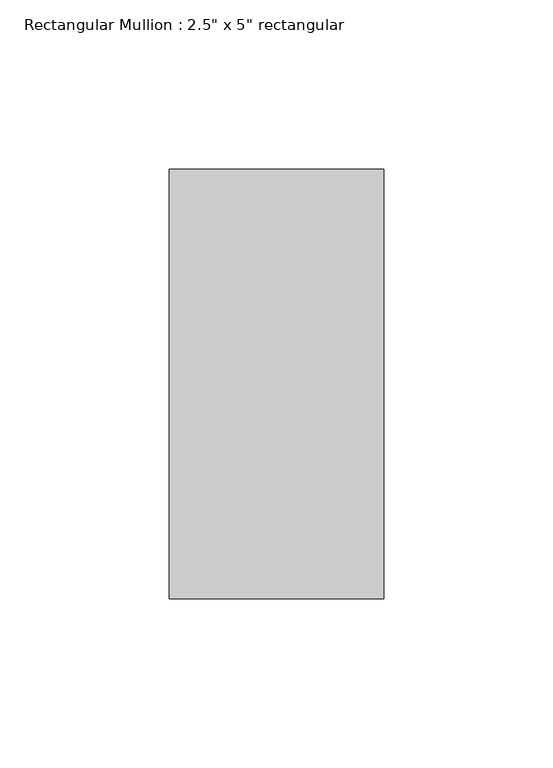
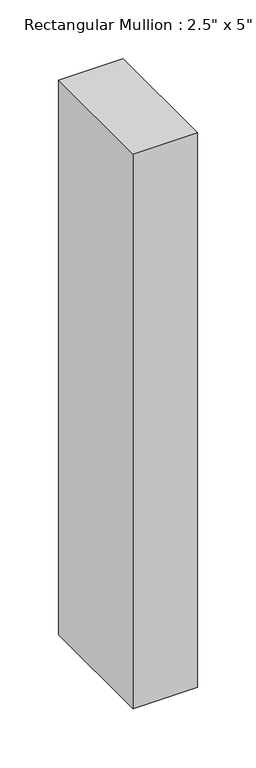
"""IFC4 building model written with IfcOpenShell, lengths in millimetres: member geometry."""

from ifc_helpers import new_model, si_unit, frame, origin, place, context, project, spatial, polyline, outline, extrude, source, transform, mapped, element, save


def member_4b1d6a2e(model_context):
    return source(origin(), model_context, "Body", "SweptSolid", [
        extrude(outline(polyline([(31.75, 63.5), (31.75, -63.5), (-31.75, -63.5), (-31.75, 63.5), (31.75, 63.5)])), frame((0.0, 0.0, -577.9826807), z_axis=(0.0, 0.0, 1.0), x_axis=(1.0, 0.0, 0.0)), (0.0, 0.0, 1.0), 577.9826807),
    ])


if __name__ == "__main__":
    model = new_model("IFC4")
    model_context = context("Model", 3, world=origin())
    ifc_project = project(units=[si_unit("LENGTHUNIT", "METRE", prefix="MILLI")], contexts=[model_context])
    site = spatial("IfcSite", under=ifc_project)
    building = spatial("IfcBuilding", under=site)
    placement = place(None, origin())
    member_shape = member_4b1d6a2e(model_context)
    element("IfcMember", 1, ObjectType="Rectangular Mullion : 2.5\" x 5\" rectangular", at=placement, inside=building, context=model_context, shape_type="MappedRepresentation", body=[
        mapped(member_shape, transform((0.0, 0.0, 0.0), x_axis=(1.0, 0.0, 0.0), y_axis=(0.0, 1.0, 0.0), z_axis=(0.0, 0.0, 1.0))),
    ])
    save(model, "model.ifc")

# Revit data of these elements
# Type "Rectangular Mullion : 2.5\" x 5\" rectangular"
#   built-in parameter 1007304 = 0.416667 (stored number, unit not read)
#   built-in parameter 1007301 = 0.104167 (stored number, unit not read)
#   built-in parameter 1007300 = 0.104167 (stored number, unit not read)
# Element 1 (IfcMember, "Rectangular Mullion : 2.5\" x 5\" rectangular")
#   Materials on its faces: "Aluminum"
# Materials
#   "Aluminum": class "Metal", colour RGB 247 247 247, transparency 0, Description = "Aluminum 6061", Cost = 0
